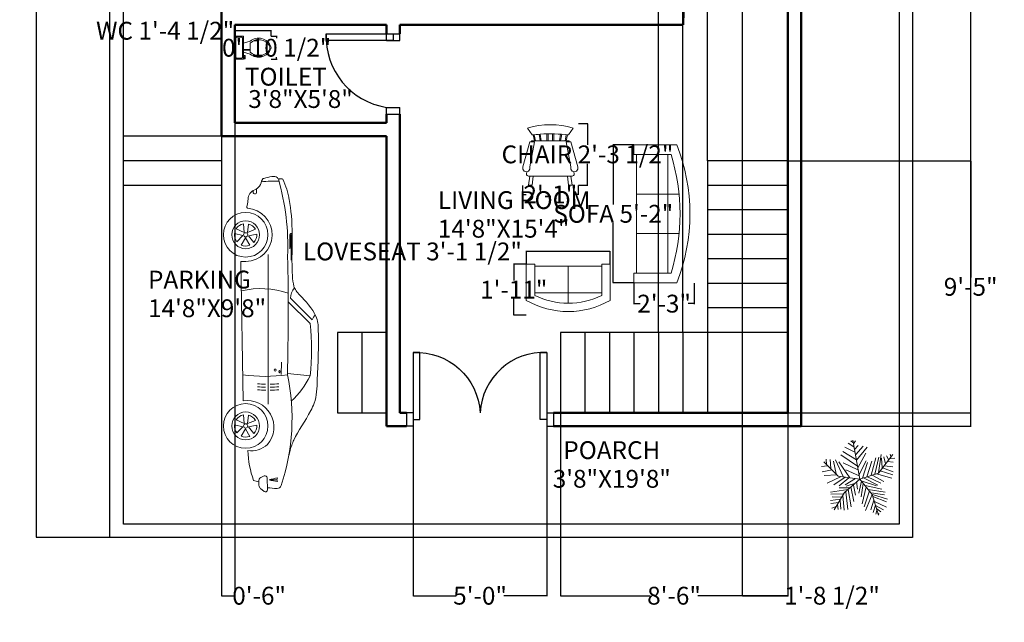
# Model space of a CAD drawing. Units: inches. Extents: x -1912 to -1462, y -785 to -198.
# Tile 1 of 3: x -1912 to -1470, y -785 to -515. Entities that reach past the tile are written whole.
import ezdxf
from ezdxf.enums import TextEntityAlignment as Align

# ---------------------------------------------------------------- set-up
doc = ezdxf.new("R2010")
doc.units = ezdxf.units.IN
doc.header["$MEASUREMENT"] = 0
for name, color, linetype, lineweight in [('A-ANNO-DIMS', 2, 'Continuous', 18), ('A-AREA-IDEN', 7, 'Continuous', 18), ('A-DOOR', 4, 'Continuous', 25), ('A-FLOR-FIXT', 8, 'Continuous', 18), ('A-FLOR-STRS', 7, 'Continuous', 25), ('A-FURN', 8, 'Continuous', 18), ('A-WALL', 7, 'Continuous', 50), ('C-PROP', 8, 'Continuous', 25), ('C-SITE-VEHI', 8, 'Continuous', 13), ('L-PLNT-TREE', 3, 'Continuous', 13)]:
    doc.layers.add(name, color=color, linetype=linetype, lineweight=lineweight)
doc.styles.get("Standard").update_dxf_attribs({"font": 'arial.ttf'})
doc.dimstyles.get("Standard").update_dxf_attribs({"dimtxt": 8, "dimasz": 0.18, "dimexe": 0.18, "dimexo": 0.0625, "dimgap": 0.09, "dimtad": 0, "dimtih": 1, "dimtoh": 1, "dimzin": 0, "dimdsep": 46, "dimlunit": 3, "dimtxsty": 'Standard', "dimcen": 0.09, "dimadec": 0, "dimazin": 0, "dimtfac": 1, "dimtofl": 0, "dimtmove": 0, "dimatfit": 3, "dimfxl": 1, "dimtolj": 1, "dimtzin": 0, "dimarcsym": 0})

# ---------------------------------------------------------------- blocks, each defined once
blk = doc.blocks.new('Chair - Rocking')
for p, q in [((-8, -4.5), (-10, -1.5)), ((-4.5, -7), (-4.96674, -4.19951)), ((-4, -7), (-4.40532, -4.16272)), ((-1.5, -4.05012), (-1.5, -7)), ((-1, -7), (-1, -4.05012)), ((1, -7), (1, -4.04655)), ((1.5, -4.05012), (1.5, -7)), ((4, -7), (4.40187, -4.18694)), ((4.5, -7), (4.96761, -4.19437)), ((8, -4.5), (10, -1.5)), ((-9, -7.5), (-12, -18.49999)), ((-7, -7.5), (-9, -7.5)), ((-9, -18.49999), (-7, -7.5)), ((-8.23428, -6.99939), (-8.3093, -7.47958)), ((-8.23041, -7), (8.23915, -7)), ((-7.5, -4.5), (-7, -7)), ((-6.5, -7), (-7.02225, -4.43)), ((6.5, -7), (7, -4.4057)), ((7.5, -4.5), (7, -7)), ((7, -7.5), (9, -7.5)), ((9, -18.49999), (7, -7.5)), ((8.31071, -7.48854), (8.23449, -7.00073)), ((9, -7.5), (12, -18.49999)), ((-10.36644, -20.64523), (-10.5, -21.49999)), ((10.5, -21.49999), (10.3575, -20.58798)), ((-9, -22.49999), (-9.5, -26.49999)), ((0, -22.49999), (-9.5, -22.49999)), ((-8, -26.49999), (-7.5, -22.49999)), ((0, -22.49999), (9.5, -22.49999)), ((8, -26.49999), (7.5, -22.49999)), ((9, -22.49999), (9.5, -26.49999)), ((-9.5, -26.49999), (-8, -26.49999)), ((9.5, -26.49999), (8, -26.49999))]:
    blk.add_line(p, q)
for centre, radius, start, end in [((0, -34.08333), 34.08333, 72.93847, 107.0615), ((0, -68.25004), 64.25, 93.92211, 97.15267), ((0, -68.25004), 64.25, 82.84733, 93.92211), ((-10.5, -18.99999), 1.58114, 161.5651, 18.43495), ((-9.5, -21.49999), 1, 180, 270), ((10.5, -18.99999), 1.58114, 161.5651, 18.43495), ((9.5, -21.49999), 1, 270, 0)]:
    blk.add_arc(centre, radius, start, end)
blk = doc.blocks.new('Sofa - Roundback Loveseat 5 ft.')
for p, q in [((0, -32.44198), (0, -5.99998)), ((-24, -33.99998), (-24, -11.46958)), ((-23.9998, -13.38178), (23.99986, -13.38178)), ((24.00004, -33.99998), (24.00004, -11.46958)), ((-24, -32.44198), (24.00004, -32.44198))]:
    blk.add_line(p, q)
for points in [[(-24, -33.99998), (-30, -33.99998), (-30, -7.99998)], [(30.00004, -7.99998), (30.00004, -33.99998), (24.00004, -33.99998)]]:
    blk.add_lwpolyline(points)
for centre, radius, start, end in [((0, -60.24998), 60.24998, 60.13715, 119.8628), ((0, -61.38438), 55.38444, 64.32083, 115.6792)]:
    blk.add_arc(centre, radius, start, end)
blk = doc.blocks.new('Sofa - Roundback 7 ft.')
for p, q in [((-36.000027, -34), (-36.000027, -11.4696)), ((-12.00002, -32.4421), (-12.00003, -6.5971)), ((11.99997, -32.4421), (11.99998, -6.5971)), ((35.99998, -34), (35.99998, -11.4696)), ((-35.999844, -13.3819), (35.9998, -13.3819)), ((-36.000027, -32.4421), (35.99998, -32.4421))]:
    blk.add_line(p, q)
for points in [[(-36.000027, -34), (-42.000027, -34), (-42.000027, -8)], [(41.99998, -8), (41.99998, -34), (35.99998, -34)]]:
    blk.add_lwpolyline(points)
for centre, radius, start, end in [((0, -114.25), 114.25, 68.43141, 111.5686), ((-0.00001, -127.1968), 121.1968, 72.72033, 107.2797)]:
    blk.add_arc(centre, radius, start, end)
blk = doc.blocks.new('Toilet - top')
for p, q in [((-10, -8.5), (-8, -8.5)), ((-10, -9.5), (-10, -8.5)), ((-8, -8.5), (-8, -8)), ((-7, -8), (-7, -9.5)), ((-4, -8), (-6, -14)), ((4, -8), (6, -14)), ((9.5, -6), (9.5, -2)), ((-7, -9.5), (-10, -9.5)), ((4, -14), (-4, -14))]:
    blk.add_line(p, q)
blk.add_lwpolyline([(10.5, -8), (10.5, 0), (-10.5, 0), (-10.5, -8)], close=True)
for points in [[(-9.5, -2), (-9.5, -6)], [(8.5, -1), (-8.5, -1)], [(-8.5, -7), (8.5, -7)]]:
    blk.add_lwpolyline(points)
for centre, radius, start, end in [((-8.62, -1.88), 0.884, 81.8699, 188.1301), ((-8.62, -6.12), 0.884, 171.8699, 278.1301), ((8.62, -1.88), 0.884, 351.8699, 98.1301), ((8.62, -6.12), 0.884, 261.8699, 8.1301), ((3.52, -21.58), 12.17, 141.46911, 247.97143), ((4.2, -21.82), 11.33, 136.36773, 238.94682), ((-3.52, -21.58), 12.17, 292.02843, 38.53071), ((-4.2, -21.82), 11.33, 301.05301, 43.63209), ((0, -27.88), 4, 245.73182, 294.26817), ((0, -29), 4, 254.86053, 285.13947)]:
    blk.add_arc(centre, radius, start, end)
blk = doc.blocks.new('*U9')
for p, q in [((1852, 1022), (2179, 1351)), ((1905, 986), (2237, 1320)), ((3032, 1318), (2995, 973)), ((1273, 1043), (872, 1041)), ((1099, 1012), (893, 1010)), ((897, 1028), (1273, 1032)), ((2822, 882), (3009, 880)), ((1185, 681), (3462, 680)), ((4554, 619), (4578, 571)), ((4581, 665), (4763, 671)), ((4742, 563), (4788, 619)), ((189, 502), (247, 503)), ((248, 455), (217, 455)), ((263, 487), (264, 471)), ((4639, 537), (4697, 540)), ((1292, 344), (1293, 267))]:
    blk.add_line(p, q)
for points in [[(897, 1014), (897, 1023, 0.269532), (893, 1030), (873, 1041, 0.575383), (867, 1037), (868, 1028, 0.269532), (872, 1022), (891, 1011, 0.575383)], [(724, 383), (854, 366), (804, 487, 0.199906)], [(880, 509), (903, 380), (1003, 465, 0.199906)], [(3628, 383), (3758, 366), (3709, 487, 0.199906)], [(3784, 509), (3808, 380), (3908, 465, 0.199906)], [(795, 196), (852, 314), (721, 305, 0.199906)], [(1048, 400), (932, 338), (1044, 269, 0.199906)], [(3700, 196), (3757, 314), (3626, 305, 0.199906)], [(3952, 400), (3837, 338), (3948, 269, 0.199906)], [(995, 206), (901, 297), (870, 170, 0.199906)], [(3900, 206), (3805, 297), (3774, 170, 0.199906)]]:
    blk.add_lwpolyline(points, format="xyb", close=True)
for points in [[(4612, 698), (4611, 811), (4584, 824)], [(4612, 698), (4611, 811), (4637, 824)], [(1293, 267), (3413, 300)]]:
    blk.add_lwpolyline(points)
for centre, radius in [((2944, 788), 15.7), ((888, 339), 339), ((3793, 339), 339), ((888, 339), 212), ((3793, 339), 212), ((888, 339), 31.7), ((3793, 339), 31.7)]:
    blk.add_circle(centre, radius)
for centre, radius, start, end in [((2911, 2669), 1508, 237.6103, 240.9785), ((2628, -2413), 3754, 83.8163, 95.9705), ((2426, 99), 1362, 43.2748, 63.5665), ((1861, 1282), 261, 230.424, 268.0085), ((1071, -2828), 3808, 87.8393, 105.8096), ((522, -80), 1094, 98.5304, 116.112), ((2035, -34649), 35635, 88.423, 91.3179), ((3005, 572), 1299, 161.4307, 193.2363), ((3687, -2156), 3200, 71.5283, 102.1242), ((652, 634), 2388, 351.8279, 8.1674), ((2011, 765), 1938, 177.5773, 185.5205), ((1159, 682), 2000, 0.852, 4.6556), ((1205, 682), 2000, 0.852, 4.6556), ((1250, 683), 2000, 0.852, 4.6556), ((3812, 365), 404, 49.2263, 189.1528), ((5493, 959), 919, 188.4683, 196.5315), ((3726, 939), 919, 344.7432, 352.8063), ((4681, 819), 63.3, 357.932, 71.5283), ((2960, 881), 1785, 353.1942, 357.932), ((888, 339), 404, 0.6373, 176.3412), ((1159, 682), 2000, 355.2644, 358.8633), ((1205, 682), 2000, 355.2644, 358.8633), ((1250, 683), 2000, 355.2644, 358.8633), ((3795, 420), 377, 352.7285, 41.6613), ((4582, 633), 31.7, 91.939, 207.109), ((4764, 639), 31.7, 320.1683, 91.939), ((248, 487), 15.8, 0.6373, 90.6373), ((248, 471), 15.8, 270.6373, 0.6373), ((4127, 1799), 1427, 271.6865, 290.2774), ((4635, 600), 63.3, 207.109, 273.4677), ((2902, 940), 1785, 344.3985, 346.9385), ((4693, 604), 63.3, 273.4677, 320.1683)]:
    blk.add_arc(centre, radius, start, end)
blk.add_ellipse((2969, 853), major_axis=(-16, -0.2), ratio=0.610043)
for points, knots in [([(289, 989), (459, 1021), (785, 1067), (1645, 1019), (1784, 1141), (2092, 1432), (2519, 1455), (2948, 1431), (3379, 1419), (3689, 1267), (3902, 1113), (4094, 1033), (4189, 1009), (4249, 994)], [18.629823, 18.629823, 18.629823, 18.629823, 19.527405, 20.700571, 21.107983, 21.608568, 21.92336, 23.151359, 23.716171, 23.908743, 24.77794, 24.943072, 25.187755, 25.187755, 25.187755, 25.187755]), ([(485, 365), (482, 361), (470, 351), (390, 381), (234, 354), (184, 564), (77, 575), (34, 600), (16, 684), (-24, 800), (39, 829), (38, 865), (38, 884), (38, 890), (39, 897), (40, 902)], [16.815853, 16.815853, 16.815853, 16.815853, 16.838212, 16.885395, 17.18439, 17.479846, 17.654423, 17.670693, 17.696923, 18.016358, 18.052739, 18.140805, 18.140805, 18.140805, 18.172382, 18.172382, 18.172382, 18.172382])]:
    blk.add_open_spline(points, degree=3, knots=knots)
blk = doc.blocks.new('*U11')
for p, q in [((-7.288, 39.707), (-21.778, 46.673)), ((-8.737, 47.138), (-17.069, 52.711)), ((-10.186, 53.64), (-13.084, 55.962)), ((0, 0), (-10.5, 57)), ((-9.099, 51.782), (-6.563, 55.962)), ((-7.65, 43.423), (-2.578, 49.46)), ((-5.839, 35.992), (4.667, 48.067)), ((-5.114, 27.632), (10.463, 46.673)), ((-48.585, 21.131), (-49.309, 29.026)), ((-3.665, 19.273), (-27.574, 35.527)), ((-5.114, 28.097), (-24.676, 40.636)), ((-2.941, 16.486), (8.652, 37.85)), ((16.259, 5.805), (23.142, 31.348)), ((22.055, 7.198), (27.489, 32.277)), ((27, 9), (48, 36)), ((27.127, 9.056), (31.112, 35.992)), ((31.836, 30.883), (32.561, 16.486)), ((35.096, 32.741), (37.27, 22.524)), ((38.719, 34.134), (41.979, 28.561)), ((43.791, 29.954), (51.036, 30.883)), ((44.153, 36.456), (45.239, 32.741)), ((-47.498, 19.737), (-55.83, 18.344)), ((-31.5, 4.5), (-52.5, 25.5)), ((-43.513, 28.561), (-42.427, 15.558)), ((-38.442, 26.239), (-34.819, 7.663)), ((-35.544, 28.097), (-24.314, 3.947)), ((-14.533, 2.09), (-30.834, 25.31)), ((-24.314, 23.917), (-2.941, 13.7)), ((-1.129, 6.734), (9.014, 26.704)), ((3.942, 1.625), (11.187, 24.381)), ((10.101, 3.483), (17.708, 26.239)), ((33.285, 16.486), (48.862, 10.913)), ((36.183, 19.737), (48.137, 17.88)), ((40.53, 25.775), (48.862, 24.846)), ((-40.615, 13.7), (-55.105, 10.913)), ((-33.37, 6.269), (-52.207, 5.34)), ((-28.299, 3.483), (-47.86, -5.805)), ((-21.416, 3.018), (-38.079, -8.128)), ((0, 0), (-31.5, 4.5)), ((-15.982, 2.09), (-30.11, -9.521)), ((0, 0), (-22.5, -19.5)), ((-6.563, 1.161), (-21.416, -8.128)), ((-20.691, 13.7), (-1.129, 4.876)), ((0, 0), (27, 9)), ((0, 0), (18, -22.5)), ((6.478, 1.625), (26.04, -8.592)), ((11.187, 3.483), (30.749, -5.805)), ((18.07, 5.805), (35.096, -3.483)), ((24.229, 7.663), (46.688, 1.625)), ((29.662, 12.307), (48.137, 6.269)), ((-15.257, -12.772), (-30.11, -12.772)), ((-6.563, -5.805), (-19.967, -9.985)), ((-13.446, -11.378), (-8.737, -32.741)), ((-9.461, -8.592), (-6.201, -23.453)), ((-4.752, -3.483), (-3.665, -14.629)), ((2.493, -3.019), (-1.491, -20.202)), ((1.769, -2.555), (24.229, -9.521)), ((5.029, -6.27), (2.131, -25.775)), ((9.014, -11.378), (3.58, -35.992)), ((7.565, -9.056), (32.198, -14.629)), ((-17.431, -15.094), (-42.789, -18.809)), ((-24.314, -21.596), (-42.427, -22.06)), ((-26.849, -26.24), (-40.253, -25.775)), ((-22.5, -19.5), (-37.5, -45)), ((-25.038, -23.918), (-22.865, -45.281)), ((-20.691, -18.345), (-17.793, -44.352)), ((-17.069, -15.094), (-12.721, -40.172)), ((14.085, -16.951), (6.478, -40.172)), ((18.07, -22.524), (8.289, -45.745)), ((12.274, -15.094), (36.907, -18.809)), ((16.259, -19.738), (36.183, -22.989)), ((18, -22.5), (27, -52.5)), ((18.433, -22.524), (40.53, -29.026)), ((19.157, -25.311), (38.719, -33.206)), ((-28.299, -29.026), (-42.789, -31.348)), ((-30.834, -34.135), (-42.427, -35.528)), ((-34.457, -39.708), (-40.978, -42.494)), ((-32.646, -36.921), (-31.921, -44.352)), ((-29.023, -30.884), (-27.936, -43.887)), ((20.244, -30.419), (15.897, -44.816)), ((22.78, -37.85), (19.519, -48.532)), ((21.331, -32.741), (39.081, -40.636)), ((22.78, -38.314), (34.372, -44.816)), ((24.591, -45.745), (23.142, -50.854)), ((24.591, -43.423), (30.749, -47.603)), ((26.764, -49.925), (28.213, -50.854))]:
    blk.add_line(p, q)
blk = doc.blocks.new('*D13')
at = {"layer": 'A-ANNO-DIMS', "color": 0, "lineweight": -2, "transparency": 16777216}
for p, q in [((-1871.14, -267.24), (-1904.18, -267.24)), ((-1904, -267.42), (-1904, -503.07)), ((-1904, -747.06), (-1904, -511.42)), ((-1871.14, -747.24), (-1904.18, -747.24))]:
    blk.add_line(p, q, dxfattribs=at)
at = {"layer": 'A-ANNO-DIMS', "color": 0, "transparency": 16777216}
for points in [[(-1904.03, -267.42), (-1903.97, -267.42), (-1904, -267.24)], [(-1904.03, -747.06), (-1903.97, -747.06), (-1904, -747.24)]]:
    blk.add_solid(points, dxfattribs=at)
at = {"layer": 'Defpoints', "color": 0, "transparency": 16777216}
for p in [(-1871.08, -267.24), (-1904, -747.24), (-1871.08, -747.24)]:
    blk.add_point(p, dxfattribs=at)
at = {"layer": 'A-ANNO-DIMS', "color": 0, "transparency": 16777216, "insert": (-1904, -507.24), "char_height": 8, "attachment_point": 5}
blk.add_mtext("\\A1;40'", dxfattribs=at)
blk = doc.blocks.new('DOOR-30IN-LEAF-HINGE-JAMB')
for p, q in [((0, 3), (0, -3)), ((0, 3), (3, 3)), ((3, 3), (3, -3)), ((0, -3), (3, -3))]:
    blk.add_line(p, q)
blk.add_lwpolyline([(0, 0), (-3, 0), (-3, 30), (0, 30)], close=True)
blk.add_arc((-1.5, 1.5), 28.54, 86.9872, 176.9872)
blk = doc.blocks.new('*D19')
at = {"layer": 'A-ANNO-DIMS', "color": 0, "lineweight": -2, "transparency": 16777216}
for p, q in [((-1815.08, -519.88), (-1815.26, -519.88)), ((-1815.08, -522.26), (-1815.08, -519.7)), ((-1798.96, -519.88), (-1814.9, -519.88)), ((-1798.78, -522.26), (-1798.78, -519.7))]:
    blk.add_line(p, q, dxfattribs=at)
at = {"layer": 'A-ANNO-DIMS', "color": 0, "transparency": 16777216}
for points in [[(-1814.9, -519.85), (-1814.9, -519.91), (-1815.08, -519.88)], [(-1798.96, -519.85), (-1798.96, -519.91), (-1798.78, -519.88)]]:
    blk.add_solid(points, dxfattribs=at)
at = {"layer": 'Defpoints', "color": 0, "transparency": 16777216}
for p in [(-1815.08, -519.88), (-1815.08, -522.32), (-1798.78, -522.32)]:
    blk.add_point(p, dxfattribs=at)
at = {"layer": 'A-ANNO-DIMS', "color": 0, "transparency": 16777216, "insert": (-1846.33, -519.88), "char_height": 8, "attachment_point": 5}
blk.add_mtext('\\A1;WC 1\'-4 1/2"', dxfattribs=at)
blk = doc.blocks.new('*D20')
at = {"layer": 'A-ANNO-DIMS', "color": 0, "lineweight": -2, "transparency": 16777216}
for p, q in [((-1798.71, -522.32), (-1796.15, -522.32)), ((-1796.33, -522.5), (-1796.33, -523.27)), ((-1798.71, -532.68), (-1796.15, -532.68)), ((-1796.33, -532.5), (-1796.33, -531.73))]:
    blk.add_line(p, q, dxfattribs=at)
at = {"layer": 'A-ANNO-DIMS', "color": 0, "transparency": 16777216}
for points in [[(-1796.36, -522.5), (-1796.3, -522.5), (-1796.33, -522.32)], [(-1796.36, -532.5), (-1796.3, -532.5), (-1796.33, -532.68)]]:
    blk.add_solid(points, dxfattribs=at)
at = {"layer": 'Defpoints', "color": 0, "transparency": 16777216}
for p in [(-1798.78, -522.32), (-1796.33, -522.32), (-1798.78, -532.68)]:
    blk.add_point(p, dxfattribs=at)
at = {"layer": 'A-ANNO-DIMS', "color": 0, "transparency": 16777216, "insert": (-1796.33, -527.5), "char_height": 8, "attachment_point": 5}
blk.add_mtext('\\A1;0\'-10 1/2"', dxfattribs=at)
blk = doc.blocks.new('*D21')
at = {"layer": 'A-ANNO-DIMS', "color": 0, "lineweight": -2, "transparency": 16777216}
for p, q in [((-1660.99, -561.52), (-1656.72, -561.52)), ((-1656.9, -561.7), (-1656.9, -571.12)), ((-1656.9, -588.99), (-1656.9, -579.57)), ((-1660.99, -589.17), (-1656.72, -589.17))]:
    blk.add_line(p, q, dxfattribs=at)
at = {"layer": 'A-ANNO-DIMS', "color": 0, "transparency": 16777216}
for points in [[(-1656.93, -561.7), (-1656.87, -561.7), (-1656.9, -561.52)], [(-1656.93, -588.99), (-1656.87, -588.99), (-1656.9, -589.17)]]:
    blk.add_solid(points, dxfattribs=at)
at = {"layer": 'Defpoints', "color": 0, "transparency": 16777216}
for p in [(-1661.05, -561.52), (-1656.9, -561.52), (-1661.05, -589.17)]:
    blk.add_point(p, dxfattribs=at)
at = {"layer": 'A-ANNO-DIMS', "color": 0, "transparency": 16777216, "insert": (-1656.9, -575.34), "char_height": 8, "attachment_point": 5}
blk.add_mtext('\\A1;CHAIR 2\'-3 1/2"', dxfattribs=at)
blk = doc.blocks.new('*D22')
at = {"layer": 'A-ANNO-DIMS', "color": 0, "lineweight": -2, "transparency": 16777216}
for p, q in [((-1686.08, -589.23), (-1686.08, -593.5)), ((-1661.05, -589.23), (-1661.05, -593.5)), ((-1685.9, -593.32), (-1684.35, -593.32)), ((-1661.23, -593.32), (-1662.77, -593.32))]:
    blk.add_line(p, q, dxfattribs=at)
at = {"layer": 'A-ANNO-DIMS', "color": 0, "transparency": 16777216}
for points in [[(-1685.9, -593.29), (-1685.9, -593.35), (-1686.08, -593.32)], [(-1661.23, -593.29), (-1661.23, -593.35), (-1661.05, -593.32)]]:
    blk.add_solid(points, dxfattribs=at)
at = {"layer": 'Defpoints', "color": 0, "transparency": 16777216}
for p in [(-1686.08, -589.17), (-1661.05, -589.17), (-1661.05, -593.32)]:
    blk.add_point(p, dxfattribs=at)
at = {"layer": 'A-ANNO-DIMS', "color": 0, "transparency": 16777216, "insert": (-1673.56, -593.32), "char_height": 8, "attachment_point": 5}
blk.add_mtext('\\A1;2\'-1"', dxfattribs=at)
blk = doc.blocks.new('*D23')
at = {"layer": 'A-ANNO-DIMS', "color": 0, "lineweight": -2, "transparency": 16777216}
for p, q in [((-1684.33, -618.88), (-1684.51, -618.88)), ((-1684.33, -624.46), (-1684.33, -618.7)), ((-1646.91, -618.88), (-1684.15, -618.88)), ((-1646.73, -624.46), (-1646.73, -618.7))]:
    blk.add_line(p, q, dxfattribs=at)
at = {"layer": 'A-ANNO-DIMS', "color": 0, "transparency": 16777216}
for points in [[(-1684.15, -618.85), (-1684.15, -618.91), (-1684.33, -618.88)], [(-1646.91, -618.85), (-1646.91, -618.91), (-1646.73, -618.88)]]:
    blk.add_solid(points, dxfattribs=at)
at = {"layer": 'Defpoints', "color": 0, "transparency": 16777216}
for p in [(-1684.33, -618.88), (-1684.33, -624.52), (-1646.73, -624.52)]:
    blk.add_point(p, dxfattribs=at)
at = {"layer": 'A-ANNO-DIMS', "color": 0, "transparency": 16777216, "insert": (-1735.43, -618.88), "char_height": 8, "attachment_point": 5}
blk.add_mtext('\\A1;LOVESEAT 3\'-1 1/2"', dxfattribs=at)
blk = doc.blocks.new('*D24')
at = {"layer": 'A-ANNO-DIMS', "color": 0, "lineweight": -2, "transparency": 16777216}
for p, q in [((-1684.39, -624.52), (-1690.15, -624.52)), ((-1689.97, -624.7), (-1689.97, -631.91)), ((-1689.97, -647.32), (-1689.97, -640.12)), ((-1684.39, -647.5), (-1690.15, -647.5))]:
    blk.add_line(p, q, dxfattribs=at)
at = {"layer": 'A-ANNO-DIMS', "color": 0, "transparency": 16777216}
for points in [[(-1690, -624.7), (-1689.94, -624.7), (-1689.97, -624.52)], [(-1690, -647.32), (-1689.94, -647.32), (-1689.97, -647.5)]]:
    blk.add_solid(points, dxfattribs=at)
at = {"layer": 'Defpoints', "color": 0, "transparency": 16777216}
for p in [(-1684.33, -624.52), (-1689.97, -647.5), (-1684.33, -647.5)]:
    blk.add_point(p, dxfattribs=at)
at = {"layer": 'A-ANNO-DIMS', "color": 0, "transparency": 16777216, "insert": (-1689.97, -636.01), "char_height": 8, "attachment_point": 5}
blk.add_mtext('\\A1;1\'-11"', dxfattribs=at)
blk = doc.blocks.new('*D25')
at = {"layer": 'A-ANNO-DIMS', "color": 0, "lineweight": -2, "transparency": 16777216}
for p, q in [((-1636.11, -571.01), (-1645.52, -571.01)), ((-1645.34, -571.19), (-1645.34, -597.77)), ((-1645.34, -632.81), (-1645.34, -606.23)), ((-1636.11, -632.99), (-1645.52, -632.99))]:
    blk.add_line(p, q, dxfattribs=at)
at = {"layer": 'A-ANNO-DIMS', "color": 0, "transparency": 16777216}
for points in [[(-1645.37, -571.19), (-1645.31, -571.19), (-1645.34, -571.01)], [(-1645.37, -632.81), (-1645.31, -632.81), (-1645.34, -632.99)]]:
    blk.add_solid(points, dxfattribs=at)
at = {"layer": 'Defpoints', "color": 0, "transparency": 16777216}
for p in [(-1636.04, -571.01), (-1645.34, -632.99), (-1636.04, -632.99)]:
    blk.add_point(p, dxfattribs=at)
at = {"layer": 'A-ANNO-DIMS', "color": 0, "transparency": 16777216, "insert": (-1645.34, -602), "char_height": 8, "attachment_point": 5}
blk.add_mtext('\\A1;SOFA 5\'-2"', dxfattribs=at)
blk = doc.blocks.new('*D26')
at = {"layer": 'A-ANNO-DIMS', "color": 0, "lineweight": -2, "transparency": 16777216}
for p, q in [((-1636.04, -633.05), (-1636.04, -642.46)), ((-1608.99, -633.05), (-1608.99, -642.46)), ((-1635.86, -642.28), (-1633.31, -642.28)), ((-1609.17, -642.28), (-1611.73, -642.28))]:
    blk.add_line(p, q, dxfattribs=at)
at = {"layer": 'A-ANNO-DIMS', "color": 0, "transparency": 16777216}
for points in [[(-1635.86, -642.25), (-1635.86, -642.31), (-1636.04, -642.28)], [(-1609.17, -642.25), (-1609.17, -642.31), (-1608.99, -642.28)]]:
    blk.add_solid(points, dxfattribs=at)
at = {"layer": 'Defpoints', "color": 0, "transparency": 16777216}
for p in [(-1636.04, -632.99), (-1608.99, -632.99), (-1608.99, -642.28)]:
    blk.add_point(p, dxfattribs=at)
at = {"layer": 'A-ANNO-DIMS', "color": 0, "transparency": 16777216, "insert": (-1622.52, -642.28), "char_height": 8, "attachment_point": 5}
blk.add_mtext('\\A1;2\'-3"', dxfattribs=at)
blk = doc.blocks.new('*D34')
at = {"layer": 'A-ANNO-DIMS', "color": 0, "lineweight": -2, "transparency": 16777216}
for p, q in [((-1561.02, -317.24), (-1484.85, -317.24)), ((-1485.03, -317.42), (-1485.03, -503.06)), ((-1485.03, -697.06), (-1485.03, -511.42)), ((-1561.02, -697.24), (-1484.85, -697.24))]:
    blk.add_line(p, q, dxfattribs=at)
at = {"layer": 'A-ANNO-DIMS', "color": 0, "transparency": 16777216}
for points in [[(-1485.06, -317.42), (-1485, -317.42), (-1485.03, -317.24)], [(-1485.06, -697.06), (-1485, -697.06), (-1485.03, -697.24)]]:
    blk.add_solid(points, dxfattribs=at)
at = {"layer": 'Defpoints', "color": 0, "transparency": 16777216}
for p in [(-1561.08, -317.24), (-1561.08, -697.24), (-1485.03, -697.24)]:
    blk.add_point(p, dxfattribs=at)
at = {"layer": 'A-ANNO-DIMS', "color": 0, "transparency": 16777216, "insert": (-1485.03, -507.24), "char_height": 8, "attachment_point": 5}
blk.add_mtext('\\A1;31\'-8"', dxfattribs=at)
blk = doc.blocks.new('*D35')
at = {"layer": 'A-ANNO-DIMS', "color": 0, "lineweight": -2, "transparency": 16777216}
for p, q in [((-1815.08, -561.3), (-1815.08, -773.47)), ((-1821.08, -567.3), (-1821.08, -773.47)), ((-1820.9, -773.29), (-1815.26, -773.29)), ((-1815.08, -773.29), (-1814.9, -773.29))]:
    blk.add_line(p, q, dxfattribs=at)
at = {"layer": 'A-ANNO-DIMS', "color": 0, "transparency": 16777216}
for points in [[(-1820.9, -773.26), (-1820.9, -773.32), (-1821.08, -773.29)], [(-1815.26, -773.26), (-1815.26, -773.32), (-1815.08, -773.29)]]:
    blk.add_solid(points, dxfattribs=at)
at = {"layer": 'Defpoints', "color": 0, "transparency": 16777216}
for p in [(-1815.08, -561.24), (-1821.08, -567.24), (-1815.08, -773.29)]:
    blk.add_point(p, dxfattribs=at)
at = {"layer": 'A-ANNO-DIMS', "color": 0, "transparency": 16777216, "insert": (-1804.18, -773.29), "char_height": 8, "attachment_point": 5}
blk.add_mtext('\\A1;0\'-6"', dxfattribs=at)
blk = doc.blocks.new('*D36')
at = {"layer": 'A-ANNO-DIMS', "color": 0, "lineweight": -2, "transparency": 16777216}
for p, q in [((-1669.08, -691.3), (-1669.08, -773.47)), ((-1567.08, -691.3), (-1567.08, -773.47)), ((-1668.9, -773.29), (-1628.81, -773.29)), ((-1567.26, -773.29), (-1607.35, -773.29))]:
    blk.add_line(p, q, dxfattribs=at)
at = {"layer": 'A-ANNO-DIMS', "color": 0, "transparency": 16777216}
for points in [[(-1668.9, -773.26), (-1668.9, -773.32), (-1669.08, -773.29)], [(-1567.26, -773.26), (-1567.26, -773.32), (-1567.08, -773.29)]]:
    blk.add_solid(points, dxfattribs=at)
at = {"layer": 'Defpoints', "color": 0, "transparency": 16777216}
for p in [(-1669.08, -691.24), (-1567.08, -691.24), (-1567.08, -773.29)]:
    blk.add_point(p, dxfattribs=at)
at = {"layer": 'A-ANNO-DIMS', "color": 0, "transparency": 16777216, "insert": (-1618.08, -773.29), "char_height": 8, "attachment_point": 5}
blk.add_mtext('\\A1;8\'-6"', dxfattribs=at)
blk = doc.blocks.new('*D37')
at = {"layer": 'A-ANNO-DIMS', "color": 0, "lineweight": -2, "transparency": 16777216}
for p, q in [((-1567.02, -578.24), (-1484.85, -578.24)), ((-1485.03, -578.42), (-1485.03, -630.57)), ((-1485.03, -691.06), (-1485.03, -638.92)), ((-1567.02, -691.24), (-1484.85, -691.24))]:
    blk.add_line(p, q, dxfattribs=at)
at = {"layer": 'A-ANNO-DIMS', "color": 0, "transparency": 16777216}
for points in [[(-1485.06, -578.42), (-1485, -578.42), (-1485.03, -578.24)], [(-1485.06, -691.06), (-1485, -691.06), (-1485.03, -691.24)]]:
    blk.add_solid(points, dxfattribs=at)
at = {"layer": 'Defpoints', "color": 0, "transparency": 16777216}
for p in [(-1567.08, -578.24), (-1567.08, -691.24), (-1485.03, -691.24)]:
    blk.add_point(p, dxfattribs=at)
at = {"layer": 'A-ANNO-DIMS', "color": 0, "transparency": 16777216, "insert": (-1485.03, -634.74), "char_height": 8, "attachment_point": 5}
blk.add_mtext('\\A1;9\'-5"', dxfattribs=at)
blk = doc.blocks.new('*D38')
at = {"layer": 'A-ANNO-DIMS', "color": 0, "lineweight": -2, "transparency": 16777216}
for p, q in [((-1603.08, -578.18), (-1603.08, -203.54)), ((-1602.9, -203.72), (-1595.8, -203.72)), ((-1567.26, -203.72), (-1574.36, -203.72)), ((-1567.08, -578.18), (-1567.08, -203.54))]:
    blk.add_line(p, q, dxfattribs=at)
at = {"layer": 'A-ANNO-DIMS', "color": 0, "transparency": 16777216}
for points in [[(-1602.9, -203.69), (-1602.9, -203.75), (-1603.08, -203.72)], [(-1567.26, -203.69), (-1567.26, -203.75), (-1567.08, -203.72)]]:
    blk.add_solid(points, dxfattribs=at)
at = {"layer": 'Defpoints', "color": 0, "transparency": 16777216}
for p in [(-1567.08, -203.72), (-1603.08, -578.24), (-1567.08, -578.24)]:
    blk.add_point(p, dxfattribs=at)
at = {"layer": 'A-ANNO-DIMS', "color": 0, "transparency": 16777216, "insert": (-1585.08, -203.72), "char_height": 8, "attachment_point": 5}
blk.add_mtext('\\A1;3\'-0"', dxfattribs=at)
blk = doc.blocks.new('*D39')
at = {"layer": 'A-ANNO-DIMS', "color": 0, "lineweight": -2, "transparency": 16777216}
for p, q in [((-1625.08, -655.18), (-1625.08, -203.54)), ((-1624.9, -203.72), (-1614.26, -203.72)), ((-1614.08, -655.18), (-1614.08, -203.54)), ((-1614.08, -203.72), (-1613.9, -203.72))]:
    blk.add_line(p, q, dxfattribs=at)
at = {"layer": 'A-ANNO-DIMS', "color": 0, "transparency": 16777216}
for points in [[(-1624.9, -203.69), (-1624.9, -203.75), (-1625.08, -203.72)], [(-1614.26, -203.69), (-1614.26, -203.75), (-1614.08, -203.72)]]:
    blk.add_solid(points, dxfattribs=at)
at = {"layer": 'Defpoints', "color": 0, "transparency": 16777216}
for p in [(-1614.08, -203.72), (-1625.08, -655.24), (-1614.08, -655.24)]:
    blk.add_point(p, dxfattribs=at)
at = {"layer": 'A-ANNO-DIMS', "color": 0, "transparency": 16777216, "insert": (-1600.07, -203.72), "char_height": 8, "attachment_point": 5}
blk.add_mtext('\\A1;0\'-11"', dxfattribs=at)
blk = doc.blocks.new('*D40')
at = {"layer": 'A-ANNO-DIMS', "color": 0, "lineweight": -2, "transparency": 16777216}
for p, q in [((-1735.08, -697.3), (-1735.08, -773.47)), ((-1675.08, -697.3), (-1675.08, -773.47)), ((-1734.9, -773.29), (-1715.8, -773.29)), ((-1675.26, -773.29), (-1694.36, -773.29))]:
    blk.add_line(p, q, dxfattribs=at)
at = {"layer": 'A-ANNO-DIMS', "color": 0, "transparency": 16777216}
for points in [[(-1734.9, -773.26), (-1734.9, -773.32), (-1735.08, -773.29)], [(-1675.26, -773.26), (-1675.26, -773.32), (-1675.08, -773.29)]]:
    blk.add_solid(points, dxfattribs=at)
at = {"layer": 'Defpoints', "color": 0, "transparency": 16777216}
for p in [(-1735.08, -697.24), (-1675.08, -697.24), (-1675.08, -773.29)]:
    blk.add_point(p, dxfattribs=at)
at = {"layer": 'A-ANNO-DIMS', "color": 0, "transparency": 16777216, "insert": (-1705.08, -773.29), "char_height": 8, "attachment_point": 5}
blk.add_mtext('\\A1;5\'-0"', dxfattribs=at)
blk = doc.blocks.new('*D42')
at = {"layer": 'A-ANNO-DIMS', "color": 0, "lineweight": -2, "transparency": 16777216}
for p, q in [((-1587.5, -385.06), (-1587.5, -773.47)), ((-1567.08, -385.06), (-1567.08, -773.47)), ((-1587.32, -773.29), (-1567.26, -773.29)), ((-1567.08, -773.29), (-1566.9, -773.29))]:
    blk.add_line(p, q, dxfattribs=at)
at = {"layer": 'A-ANNO-DIMS', "color": 0, "transparency": 16777216}
for points in [[(-1587.32, -773.26), (-1587.32, -773.32), (-1587.5, -773.29)], [(-1567.26, -773.26), (-1567.26, -773.32), (-1567.08, -773.29)]]:
    blk.add_solid(points, dxfattribs=at)
at = {"layer": 'Defpoints', "color": 0, "transparency": 16777216}
for p in [(-1587.5, -385), (-1567.08, -385), (-1567.08, -773.29)]:
    blk.add_point(p, dxfattribs=at)
at = {"layer": 'A-ANNO-DIMS', "color": 0, "transparency": 16777216, "insert": (-1547.23, -773.29), "char_height": 8, "attachment_point": 5}
blk.add_mtext('\\A1;1\'-8 1/2"', dxfattribs=at)

msp = doc.modelspace()

# ---------------------------------------------------------------- linework, layer by layer
at = {"layer": 'A-DOOR'}
for p, q in [((-1747.078, -521.241), (-1741.078, -521.241)), ((-1747.078, -524.241), (-1747.078, -521.241)), ((-1747.078, -524.241), (-1741.078, -524.241)), ((-1741.078, -524.241), (-1741.078, -521.241)), ((-1747.078, -554.241), (-1741.078, -554.241)), ((-1747.078, -557.241), (-1747.078, -554.241)), ((-1741.078, -557.241), (-1741.078, -554.241)), ((-1747.078, -557.241), (-1741.078, -557.241))]:
    msp.add_line(p, q, dxfattribs=at)
msp.add_lwpolyline([(-1744.078, -524.241), (-1774.078, -524.241), (-1774.078, -521.241), (-1744.078, -521.241)], close=True, dxfattribs=at)
msp.add_arc((-1742.245, -522.741), 31.869, 177.30219, 261.27662, dxfattribs=at)
at = {"layer": 'A-FLOR-STRS'}
for p, q in [((-1821.078, -567.241), (-1865.078, -567.241)), ((-1821.078, -567.241), (-1821.078, -589.241)), ((-1821.078, -578.241), (-1865.078, -578.241)), ((-1603.078, -578.241), (-1603.078, -691.241)), ((-1567.078, -578.241), (-1603.078, -578.241)), ((-1821.078, -589.241), (-1865.078, -589.241)), ((-1567.078, -589.241), (-1603.078, -589.241)), ((-1567.078, -600.241), (-1603.078, -600.241)), ((-1567.078, -611.241), (-1603.078, -611.241)), ((-1567.078, -622.241), (-1603.078, -622.241)), ((-1567.078, -633.241), (-1603.078, -633.241)), ((-1567.078, -644.241), (-1603.078, -644.241)), ((-1758.078, -655.241), (-1769.078, -655.241)), ((-1769.078, -655.241), (-1769.078, -691.241)), ((-1747.078, -655.241), (-1758.078, -655.241)), ((-1758.078, -655.241), (-1758.078, -691.241)), ((-1567.078, -655.241), (-1669.078, -655.241)), ((-1669.078, -655.241), (-1669.078, -691.241)), ((-1658.078, -655.241), (-1658.078, -691.241)), ((-1647.078, -655.241), (-1647.078, -691.241)), ((-1636.078, -655.241), (-1636.078, -691.241)), ((-1625.078, -655.241), (-1625.078, -691.241)), ((-1614.078, -655.241), (-1614.078, -691.241)), ((-1769.078, -691.241), (-1747.078, -691.241))]:
    msp.add_line(p, q, dxfattribs=at)
at = {"layer": 'A-WALL'}
for p, q in [((-1821.078, -567.241), (-1821.078, -317.241)), ((-1561.078, -317.241), (-1561.078, -697.241)), ((-1567.078, -323.241), (-1567.078, -691.241)), ((-1613.924, -517.241), (-1613.799, -511.241)), ((-1815.078, -517.241), (-1747.078, -517.241)), ((-1815.078, -561.241), (-1815.078, -517.241)), ((-1747.078, -521.241), (-1747.078, -517.241)), ((-1741.078, -517.241), (-1715.078, -517.241)), ((-1741.078, -521.241), (-1741.078, -517.241)), ((-1715.078, -517.241), (-1613.924, -517.241)), ((-1747.078, -561.241), (-1747.078, -557.241)), ((-1741.078, -567.241), (-1741.078, -557.241)), ((-1815.078, -561.241), (-1747.078, -561.241)), ((-1821.078, -567.241), (-1747.078, -567.241)), ((-1747.078, -567.241), (-1747.078, -697.241)), ((-1741.078, -567.241), (-1741.078, -691.241)), ((-1738.078, -691.241), (-1741.078, -691.241)), ((-1567.078, -691.241), (-1672.078, -691.241)), ((-1738.078, -697.241), (-1747.078, -697.241)), ((-1561.078, -697.241), (-1672.078, -697.241))]:
    msp.add_line(p, q, dxfattribs=at)
at = {"layer": 'C-PROP'}
for p, q in [((-1865.078, -741.241), (-1865.078, -273.241)), ((-1517.078, -273.241), (-1517.078, -741.241)), ((-1517.078, -741.241), (-1865.078, -741.241))]:
    msp.add_line(p, q, dxfattribs=at)
msp.add_lwpolyline([(-1511.078, -747.241), (-1871.078, -747.241), (-1871.078, -267.241), (-1511.078, -267.241)], close=True, dxfattribs=at)

# ---------------------------------------------------------------- block references
at = {"layer": 'A-DOOR', "extrusion": (0, 0, -1), "zscale": -1}
msp.add_blockref('DOOR-30IN-LEAF-HINGE-JAMB', (1735.078, -694.241), dxfattribs=at)
at = {"layer": 'A-DOOR'}
msp.add_blockref('DOOR-30IN-LEAF-HINGE-JAMB', (-1675.078, -694.241), dxfattribs=at)
at = {"layer": 'A-FLOR-FIXT', "xscale": 0.4932980712565927, "yscale": 0.4932980712565927, "zscale": 0.4932980712565927, "rotation": 90}
msp.add_blockref('Toilet - top', (-1815.078, -527.5), dxfattribs=at)
at = {"layer": 'A-FURN', "xscale": 1.024246404759472, "yscale": 1.024246404759472, "zscale": 1.024246404759472}
msp.add_blockref('Chair - Rocking', (-1673.561, -562.03), dxfattribs=at)
at = {"layer": 'A-FURN'}
for name, p, xscale, yscale, zscale, rotation in [('Sofa - Roundback 7 ft.', (-1610.959, -602), 0.7378101803215956, 0.7378101803215956, 0.7378101803215956, 270), ('Sofa - Roundback Loveseat 5 ft.', (-1665.53, -645.832), 0.6267106559430373, 0.6267106559430373, 0.6267106559430373, 180)]:
    msp.add_blockref(name, p, dxfattribs=dict(at, xscale=xscale, yscale=yscale, zscale=zscale, rotation=rotation))
at = {"layer": 'C-SITE-VEHI', "xscale": 0.0295080337495162, "yscale": 0.0295080337495162, "zscale": 0.0295080337495162, "rotation": 270}
msp.add_blockref('*U9', (-1820.222, -585.21), dxfattribs=at)
at = {"layer": 'L-PLNT-TREE', "xscale": 0.307023879819639, "yscale": 0.307023879819639, "zscale": 0.307023879819639}
msp.add_blockref('*U11', (-1534.729, -721.031), dxfattribs=at)

# ---------------------------------------------------------------- texts
at = {"layer": 'A-AREA-IDEN'}
for s, p in [('TOILET', (-1810.57, -544.5)), ('3\'8"X5\'8"', (-1809.054, -554.516)), ('LIVING ROOM', (-1724.013, -599.845)), ('14\'8"X15\'4"', (-1724.013, -612.697)), ('PARKING', (-1854, -635.5)), ('14\'8"X9\'8"', (-1854, -648.351))]:
    msp.add_text(s, height=8, dxfattribs=at).set_placement(p)
for s, p in [('POARCH', (-1646, -712)), ('3\'8"X19\'8"', (-1646, -724.851))]:
    msp.add_text(s, height=8, dxfattribs=at).set_placement(p, align=Align.CENTER)

# ---------------------------------------------------------------- dimensions: what is measured, and where the dimension line sits
at = {"layer": 'A-ANNO-DIMS'}
for base, p1, p2, picture, middle in [((-1614.078, -203.718), (-1625.078, -655.241), (-1614.078, -655.241), '*D39', (-1600.068, -203.718)), ((-1567.078, -203.718), (-1603.078, -578.241), (-1567.078, -578.241), '*D38', (-1585.078, -203.718)), ((-1567.078, -773.291), (-1587.5, -385), (-1567.078, -385), '*D42', (-1547.231, -773.291)), ((-1815.078, -773.291), (-1821.078, -567.241), (-1815.078, -561.241), '*D35', (-1804.175, -773.291)), ((-1661.048, -593.32), (-1686.075, -589.172), (-1661.048, -589.172), '*D22', (-1673.561, -593.32)), ((-1608.992, -642.284), (-1636.045, -632.988), (-1608.992, -632.988), '*D26', (-1622.518, -642.284)), ((-1567.078, -773.291), (-1669.078, -691.241), (-1567.078, -691.241), '*D36', (-1618.078, -773.291)), ((-1675.078, -773.291), (-1735.078, -697.241), (-1675.078, -697.241), '*D40', (-1705.078, -773.291))]:
    dim = msp.add_linear_dim(base=base, p1=p1, p2=p2, dimstyle='Standard', override={"dimdec": 1, "dimlfac": 1, "dimrnd": 0, "dimzin": 1, "dimdsep": 46, "dimlunit": 4, "dimfrac": 2}, dxfattribs=at)
    dim.commit()
    dim.dimension.update_dxf_attribs({"geometry": picture, "text_midpoint": middle})
for base, p1, p2, angle, override, picture, middle in [((-1904, -747.241), (-1871.078, -267.241), (-1871.078, -747.241), 90, {"dimclrd": 0, "dimclre": 0, "dimclrt": 0}, '*D13', (-1904, -507.241)), ((-1485.028, -697.241), (-1561.078, -317.241), (-1561.078, -697.241), 90, {"dimdec": 1, "dimlfac": 1, "dimrnd": 0, "dimzin": 1, "dimdsep": 46, "dimlunit": 4, "dimfrac": 2}, '*D34', (-1485.028, -507.241)), ((-1796.331, -522.32), (-1798.777, -532.68), (-1798.777, -522.32), 90, {"dimdec": 1, "dimlfac": 1, "dimrnd": 0, "dimzin": 1, "dimdsep": 46, "dimlunit": 4, "dimfrac": 2}, '*D20', (-1796.331, -527.5)), ((-1485.028, -691.241), (-1567.078, -578.241), (-1567.078, -691.241), 90, {"dimdec": 1, "dimlfac": 1, "dimrnd": 0, "dimzin": 1, "dimdsep": 46, "dimlunit": 4, "dimfrac": 2}, '*D37', (-1485.028, -634.741)), ((-1689.972, -647.503), (-1684.332, -624.524), (-1684.332, -647.503), 270, {"dimdec": 1, "dimlfac": 1, "dimrnd": 0, "dimzin": 1, "dimdsep": 46, "dimlunit": 4, "dimfrac": 2}, '*D24', (-1689.972, -636.013))]:
    dim = msp.add_linear_dim(base=base, p1=p1, p2=p2, angle=angle, dimstyle='Standard', override=override, dxfattribs=at)
    dim.commit()
    dim.dimension.update_dxf_attribs({"geometry": picture, "text_midpoint": middle})
for base, p1, p2, angle, text, picture, middle in [((-1815.078, -519.875), (-1798.777, -522.32), (-1815.078, -522.32), 180, 'WC <>', '*D19', (-1846.328, -519.875)), ((-1656.899, -561.518), (-1661.048, -589.172), (-1661.048, -561.518), 90, 'CHAIR <>', '*D21', (-1656.899, -575.345)), ((-1645.341, -632.988), (-1636.045, -571.012), (-1636.045, -632.988), 270, 'SOFA <>', '*D25', (-1645.341, -602)), ((-1684.332, -618.883), (-1646.729, -624.524), (-1684.332, -624.524), 180, 'LOVESEAT <>', '*D23', (-1735.434, -618.883))]:
    dim = msp.add_linear_dim(base=base, p1=p1, p2=p2, angle=angle, text=text, dimstyle='Standard', override={"dimdec": 1, "dimlfac": 1, "dimrnd": 0, "dimzin": 1, "dimdsep": 46, "dimlunit": 4, "dimfrac": 2}, dxfattribs=at)
    dim.commit()
    dim.dimension.update_dxf_attribs({"geometry": picture, "text_midpoint": middle})

doc.saveas('drawing.dxf')
